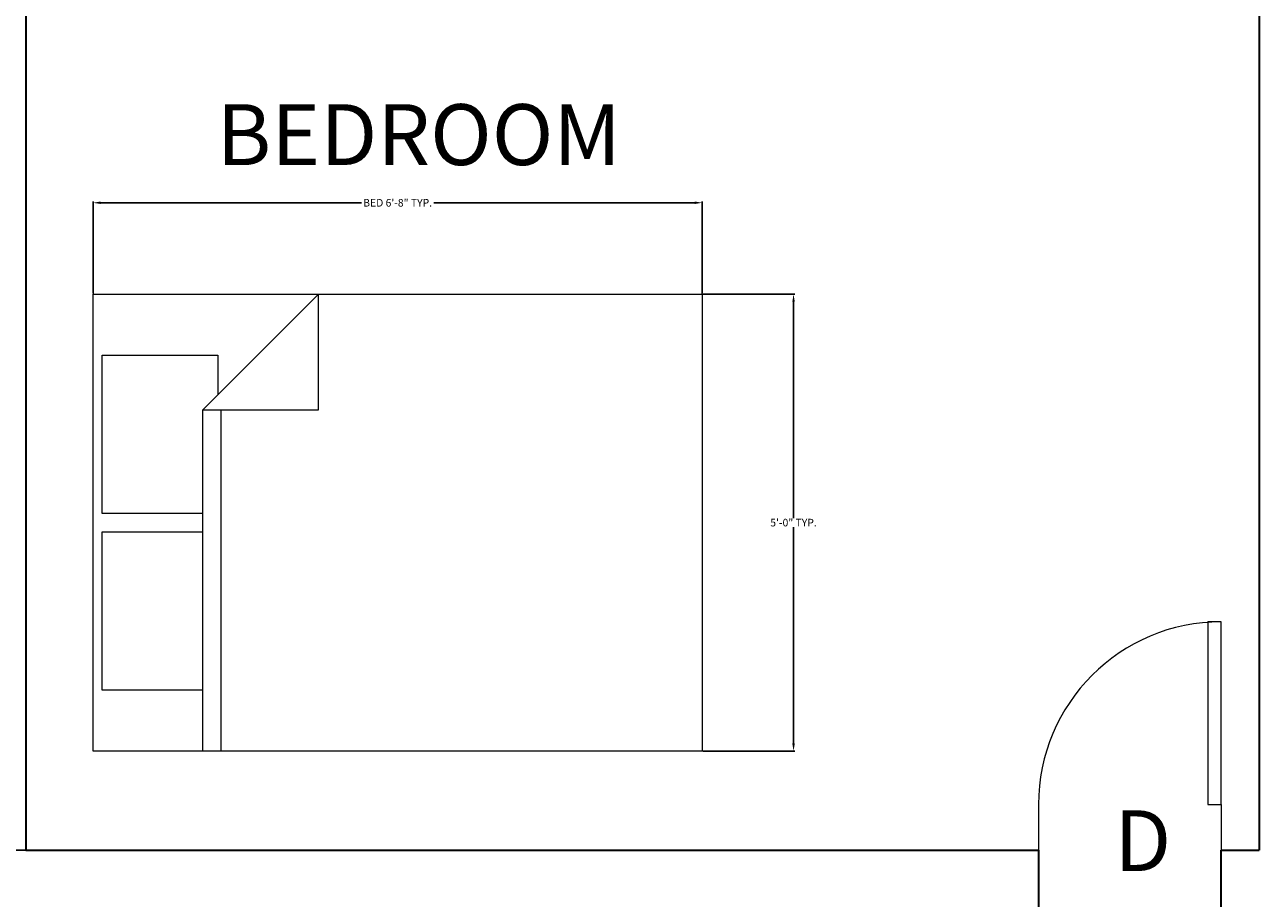
# Model space of a CAD drawing. Units: inches. Extents: x 371 to 1095, y -45 to 1219.
# Tile 15 of 18: x 502 to 664, y 799 to 913. Entities that reach past the tile are written whole.
import ezdxf

# ---------------------------------------------------------------- set-up
doc = ezdxf.new("R2010")
doc.units = ezdxf.units.IN
doc.header["$MEASUREMENT"] = 0
for name, color, linetype, lineweight in [('A-ANNO-DIMS', 2, 'Continuous', 18), ('A-ANNO-TEXT', 7, 'Continuous', 18), ('A-AREA-IDEN', 7, 'Continuous', 18), ('A-DOOR', 3, 'Continuous', 18), ('A-FURN', 254, 'Continuous', 18), ('A-WALL', 40, 'Continuous', 35)]:
    doc.layers.add(name, color=color, linetype=linetype, lineweight=lineweight)
doc.styles.get("Standard").update_dxf_attribs({"font": 'arial.ttf'})
doc.dimstyles.get("Standard").update_dxf_attribs({"dimtxt": 1, "dimasz": 1, "dimexe": 0.18, "dimexo": 0.0625, "dimgap": 0.09, "dimtad": 0, "dimtih": 1, "dimtoh": 1, "dimdec": 0, "dimzin": 0, "dimdsep": 46, "dimlunit": 3, "dimtxsty": 'Standard', "dimcen": 0.09, "dimadec": 0, "dimazin": 0, "dimtfac": 1, "dimtdec": 0, "dimtofl": 0, "dimtmove": 0, "dimatfit": 3, "dimfxl": 1, "dimtolj": 1, "dimtzin": 0, "dimarcsym": 0})

# ---------------------------------------------------------------- blocks, each defined once
blk = doc.blocks.new('*U4')
for p, q in [((-24, 0), (-24, -6)), ((0, 0), (0, -6))]:
    blk.add_line(p, q)
blk.add_lwpolyline([(0, 0), (0, 24), (-1.75, 24), (-1.75, 0)], close=True)
blk.add_arc((0, 0), 24, 90, 180)
blk = doc.blocks.new('*D8')
at = {"layer": 'A-ANNO-DIMS', "color": 0, "lineweight": -2, "transparency": 16777216}
for p, q in [((501.75, 973.03), (438.47, 973.03)), ((438.65, 972.03), (438.65, 896.65)), ((438.65, 806.03), (438.65, 881.4)), ((501.75, 805.03), (438.47, 805.03))]:
    blk.add_line(p, q, dxfattribs=at)
at = {"layer": 'A-ANNO-DIMS', "color": 0, "transparency": 16777216}
for points in [[(438.48, 972.03), (438.82, 972.03), (438.65, 973.03)], [(438.48, 806.03), (438.82, 806.03), (438.65, 805.03)]]:
    blk.add_solid(points, dxfattribs=at)
at = {"layer": 'Defpoints', "color": 0, "transparency": 16777216}
for p in [(501.81, 973.03), (438.65, 805.03), (501.81, 805.03)]:
    blk.add_point(p, dxfattribs=at)
at = {"layer": 'A-ANNO-DIMS', "color": 0, "transparency": 16777216, "insert": (438.65, 889.03), "char_height": 1, "attachment_point": 5}
blk.add_mtext("\\A1;{\\H15x;14'}", dxfattribs=at)
blk = doc.blocks.new('Bed - Queen')
for p, q in [((0, -80.00003), (0, 0)), ((0, 0), (59.99999, 0)), ((59.99999, 0), (59.99999, -80.00003)), ((7.99999, -1.2), (28.79998, -1.2)), ((7.99999, -14.4), (7.99999, -1.2)), ((28.79998, -1.2), (28.79998, -14.4)), ((31.19999, -1.2), (51.99999, -1.2)), ((31.19999, -14.4), (31.19999, -1.2)), ((51.99999, -1.2), (51.99999, -16.4)), ((0, -14.4), (44.8, -14.4)), ((59.99999, -29.6), (44.8, -14.4)), ((44.8, -14.4), (44.8, -29.6)), ((44.8, -16.8), (0, -16.8)), ((51.99999, -16.4), (46.79936, -16.4)), ((44.8, -29.6), (59.99999, -29.6)), ((59.99999, -80.00003), (0, -80.00003))]:
    blk.add_line(p, q)
blk = doc.blocks.new('*D34')
at = {"layer": 'A-ANNO-DIMS', "color": 0, "lineweight": -2, "transparency": 16777216}
for p, q in [((510.63, 878.12), (510.63, 890.23)), ((511.63, 890.05), (545.89, 890.05)), ((589.63, 890.05), (555.38, 890.05)), ((590.63, 878.12), (590.63, 890.23))]:
    blk.add_line(p, q, dxfattribs=at)
at = {"layer": 'A-ANNO-DIMS', "color": 0, "transparency": 16777216}
for points in [[(511.63, 890.22), (511.63, 889.89), (510.63, 890.05)], [(589.63, 890.22), (589.63, 889.89), (590.63, 890.05)]]:
    blk.add_solid(points, dxfattribs=at)
at = {"layer": 'Defpoints', "color": 0, "transparency": 16777216}
for p in [(510.63, 890.05), (510.63, 878.05), (590.63, 878.05)]:
    blk.add_point(p, dxfattribs=at)
at = {"layer": 'A-ANNO-DIMS', "color": 0, "transparency": 16777216, "insert": (550.63, 890.05), "char_height": 1, "attachment_point": 5}
blk.add_mtext('\\A1;BED 6\'-8" TYP.', dxfattribs=at)
blk = doc.blocks.new('*D35')
at = {"layer": 'A-ANNO-DIMS', "color": 0, "lineweight": -2, "transparency": 16777216}
for p, q in [((590.7, 878.05), (602.81, 878.05)), ((602.63, 877.05), (602.63, 848.65)), ((602.63, 819.05), (602.63, 847.45)), ((590.7, 818.05), (602.81, 818.05))]:
    blk.add_line(p, q, dxfattribs=at)
at = {"layer": 'A-ANNO-DIMS', "color": 0, "transparency": 16777216}
for points in [[(602.47, 877.05), (602.8, 877.05), (602.63, 878.05)], [(602.47, 819.05), (602.8, 819.05), (602.63, 818.05)]]:
    blk.add_solid(points, dxfattribs=at)
at = {"layer": 'Defpoints', "color": 0, "transparency": 16777216}
for p in [(590.63, 878.05), (602.63, 878.05), (590.63, 818.05)]:
    blk.add_point(p, dxfattribs=at)
at = {"layer": 'A-ANNO-DIMS', "color": 0, "transparency": 16777216, "insert": (602.63, 848.05), "char_height": 1, "attachment_point": 5}
blk.add_mtext('\\A1;5\'-0" TYP.', dxfattribs=at)

msp = doc.modelspace()

# ---------------------------------------------------------------- linework, layer by layer
at = {"layer": 'A-WALL'}
for p, q in [((501.81, 973.03), (501.81, 805.03)), ((663.81, 920.03), (663.81, 805.03)), ((501.81, 805.03), (634.81, 805.03)), ((634.81, 805.03), (634.81, 796.03)), ((658.81, 796.03), (658.81, 805.03)), ((658.81, 805.03), (663.81, 805.03))]:
    msp.add_line(p, q, dxfattribs=at)

# ---------------------------------------------------------------- block references
at = {"layer": 'A-DOOR'}
msp.add_blockref('*U4', (658.81, 811.03), dxfattribs=at)
at = {"layer": 'A-FURN', "rotation": 90}
msp.add_blockref('Bed - Queen', (510.63, 818.05), dxfattribs=at)

# ---------------------------------------------------------------- texts
at = {"layer": 'A-ANNO-TEXT', "insert": (644.74, 810.28), "char_height": 8, "attachment_point": 1}
msp.add_mtext_dynamic_manual_height_columns('D', width=17.4938, gutter_width=1, heights=[0], dxfattribs=at)
at = {"layer": 'A-AREA-IDEN', "insert": (526.86, 903), "char_height": 8, "attachment_point": 1}
msp.add_mtext_dynamic_manual_height_columns('BEDROOM', width=53.6318, gutter_width=1, heights=[0], dxfattribs=at)

# ---------------------------------------------------------------- dimensions: what is measured, and where the dimension line sits
at = {"layer": 'A-ANNO-DIMS'}
for base, p1, p2, angle, text, override, picture, middle in [((438.65, 805.03), (501.81, 973.03), (501.81, 805.03), 90, '{\\H15x;<>}', {"dimclrd": 0, "dimclre": 0, "dimclrt": 0}, '*D8', (438.65, 889.03)), ((510.63, 890.05), (590.63, 878.05), (510.63, 878.05), 180, 'BED <> TYP.', {"dimdec": 1, "dimlfac": 1, "dimrnd": 0, "dimzin": 1, "dimdsep": 46, "dimlunit": 4, "dimfrac": 2}, '*D34', (550.63, 890.05)), ((602.63, 878.05), (590.63, 818.05), (590.63, 878.05), 90, '<> TYP.', {"dimdec": 1, "dimlfac": 1, "dimrnd": 0, "dimzin": 1, "dimdsep": 46, "dimlunit": 4, "dimfrac": 2}, '*D35', (602.63, 848.05))]:
    dim = msp.add_linear_dim(base=base, p1=p1, p2=p2, angle=angle, text=text, dimstyle='Standard', override=override, dxfattribs=at)
    dim.commit()
    dim.dimension.update_dxf_attribs({"geometry": picture, "text_midpoint": middle})

doc.saveas('drawing.dxf')
